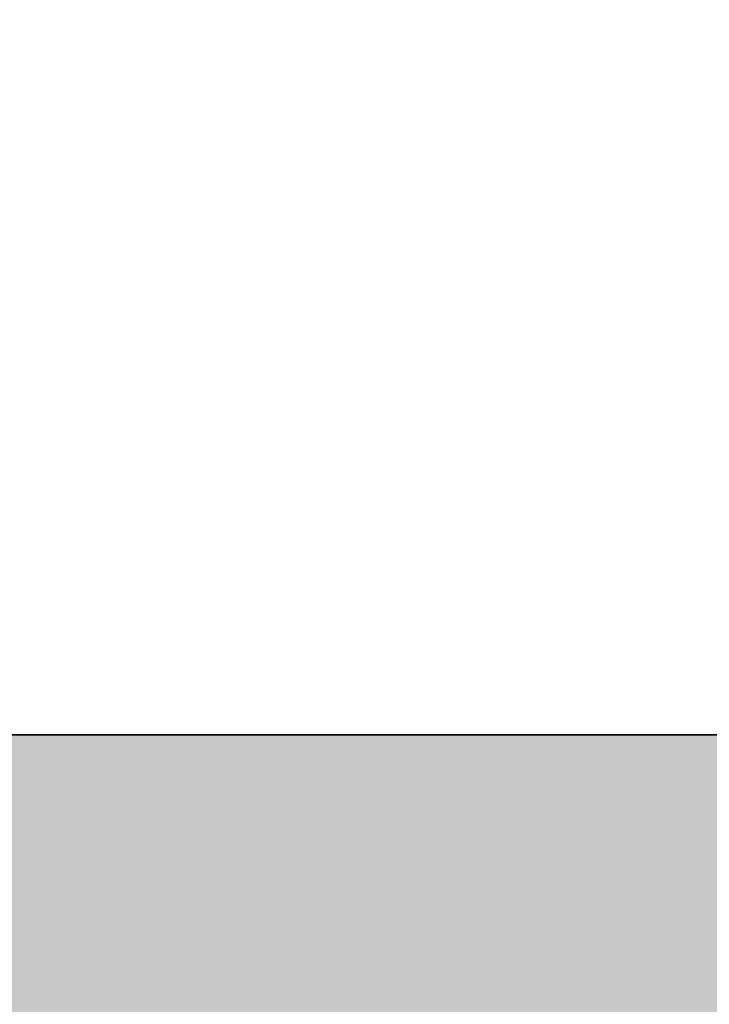
# Model space of a CAD drawing. Units: inches. Extents: x 2696 to 3240, y 1564 to 2310.
# Tile 59 of 76: x 2921.79 to 2936.43, y 2179.88 to 2200.79. Entities that reach past the tile are written whole.
import ezdxf

# ---------------------------------------------------------------- set-up
doc = ezdxf.new("R2010")
doc.units = ezdxf.units.IN
for name, color, linetype, lineweight in [('A-ANNO-DIMS', 3, 'Continuous', 18), ('A-WALL', 7, 'Continuous', 35), ('A-WALL-PATT', 9, 'Continuous', 13)]:
    doc.layers.add(name, color=color, linetype=linetype, lineweight=lineweight)
doc.styles.add('TIMES NEW', font='times.ttf')
doc.dimstyles.new('Siddhuu', dxfattribs={"dimtxt": 6, "dimasz": 2.5, "dimexe": 1.25, "dimexo": 0.625, "dimtad": 1, "dimdec": 1, "dimlunit": 4, "dimtxsty": 'TIMES NEW', "dimcen": 2.5, "dimclrd": 256, "dimclre": 1, "dimclrt": 7, "dimadec": 0, "dimazin": 0, "dimtfac": 1, "dimtdec": 1, "dimtmove": 0, "dimatfit": 3, "dimfxl": 1, "dimtolj": 1, "dimlwd": -1, "dimarcsym": 0})

# ---------------------------------------------------------------- blocks, each defined once
blk = doc.blocks.new('*D59')
at = {"layer": 'A-ANNO-DIMS', "color": 1, "lineweight": -2, "transparency": 16777216}
for p, q in [((2884.709, 1740.826), (2884.709, 2298.451)), ((2956.709, 1740.826), (2956.709, 2298.451))]:
    blk.add_line(p, q, dxfattribs=at)
at = {"layer": 'A-ANNO-DIMS', "transparency": 16777216}
blk.add_line((2887.209, 2297.201), (2954.209, 2297.201), dxfattribs=at)
for points in [[(2887.209, 2297.618), (2887.209, 2296.784), (2884.709, 2297.201)], [(2954.209, 2297.618), (2954.209, 2296.784), (2956.709, 2297.201)]]:
    blk.add_solid(points, dxfattribs=at)
at = {"layer": 'Defpoints', "color": 0, "transparency": 16777216}
for p in [(2956.709, 2297.201), (2884.709, 1740.201), (2956.709, 1740.201)]:
    blk.add_point(p, dxfattribs=at)
at = {"layer": 'A-ANNO-DIMS', "color": 7, "transparency": 16777216, "insert": (2920.709, 2300.878), "char_height": 6, "attachment_point": 5, "style": 'TIMES NEW'}
blk.add_mtext('\\A1;6\'-0"', dxfattribs=at)
blk = doc.blocks.new('*D64')
at = {"layer": 'A-ANNO-DIMS', "color": 1, "lineweight": -2, "transparency": 16777216}
for p, q in [((3073.084, 2206.701), (2709.361, 2206.701)), ((3068.584, 1989.201), (2709.361, 1989.201))]:
    blk.add_line(p, q, dxfattribs=at)
at = {"layer": 'A-ANNO-DIMS', "transparency": 16777216}
blk.add_line((2710.611, 1991.701), (2710.611, 2204.201), dxfattribs=at)
for points in [[(2710.195, 2204.201), (2711.028, 2204.201), (2710.611, 2206.701)], [(2710.195, 1991.701), (2711.028, 1991.701), (2710.611, 1989.201)]]:
    blk.add_solid(points, dxfattribs=at)
at = {"layer": 'Defpoints', "color": 0, "transparency": 16777216}
for p in [(2710.611, 2206.701), (3073.709, 2206.701), (3069.209, 1989.201)]:
    blk.add_point(p, dxfattribs=at)
at = {"layer": 'A-ANNO-DIMS', "color": 7, "transparency": 16777216, "insert": (2706.85, 2097.951), "char_height": 6, "attachment_point": 5, "rotation": 90, "style": 'TIMES NEW'}
blk.add_mtext('\\A1;18\'-1 1/2"', dxfattribs=at)

msp = doc.modelspace()

# ---------------------------------------------------------------- hatches: boundary and pattern name
at = {"layer": 'A-WALL-PATT', "transparency": 33554556}
h = msp.add_hatch(color=256, dxfattribs=at)
h.dxf.hatch_style = 1
h.paths.add_polyline_path([(2879.111, 2253.201), (2905.91, 2253.201), (2905.91, 2262.201), (2841.889, 2262.201), (2841.889, 2253.201), (2870.111, 2253.201), (2870.111, 2176.601), (2965.709, 2176.601), (2965.709, 2206.701), (2973.583, 2206.701), (2973.583, 2215.701), (2965.709, 2215.701), (2965.709, 2262.201), (2929.91, 2262.201), (2929.91, 2253.201), (2956.709, 2253.201), (2956.709, 2185.601), (2879.111, 2185.601)])
h.paths.add_polyline_path([(2782.834, 2262.201), (2745.611, 2262.201), (2745.611, 2228.729), (2754.611, 2228.729), (2754.611, 2253.201), (2782.834, 2253.201)])
h.paths.add_polyline_path([(2754.611, 2136.201), (2965.709, 2136.201), (2965.709, 2145.201), (2879.111, 2145.201), (2879.111, 2147.074), (2877.34, 2147.074), (2870.111, 2147.074), (2870.111, 2145.201), (2754.611, 2145.201), (2754.611, 2169.674), (2745.611, 2169.674), (2745.611, 2000.201), (2754.611, 2000.201), (2754.611, 2019.201), (2849.083, 2019.201), (2849.083, 2023.701), (2841.209, 2023.701), (2841.209, 2051.827), (2836.709, 2051.827), (2836.709, 2023.701), (2754.611, 2023.701), (2754.611, 2091.201), (2836.709, 2091.201), (2836.709, 2087.827), (2841.209, 2087.827), (2841.209, 2095.701), (2754.611, 2095.701)])
h.paths.add_polyline_path([(2965.709, 2136.201), (2956.709, 2136.201), (2956.709, 2023.701), (2885.083, 2023.701), (2885.083, 2019.201), (2956.709, 2019.201), (2956.709, 1950.575), (2965.709, 1950.575), (2965.709, 1980.201), (2973.583, 1980.201), (2973.583, 1989.201), (2965.709, 1989.201)])
h.paths.add_polyline_path([(2754.611, 1906.701), (2880.209, 1906.701), (2884.709, 1906.701), (2956.709, 1906.701), (2956.709, 1792.701), (2944.709, 1792.701), (2944.709, 1783.701), (2956.709, 1783.701), (2956.709, 1740.201), (2884.709, 1740.201), (2884.709, 1783.701), (2896.709, 1783.701), (2896.709, 1792.701), (2884.709, 1792.701), (2884.709, 1846.701), (2880.209, 1846.701), (2880.209, 1740.201), (2754.611, 1740.201), (2754.611, 1777.201), (2745.611, 1777.201), (2745.611, 1692.701), (2754.611, 1692.701), (2754.611, 1731.201), (2956.709, 1731.201), (2956.709, 1723.327), (2965.709, 1723.327), (2965.709, 1884.201), (2973.583, 1884.201), (2973.583, 1893.201), (2965.709, 1893.201), (2965.709, 1914.575), (2956.709, 1914.575), (2956.709, 1911.201), (2754.611, 1911.201), (2754.611, 1930.201), (2745.611, 1930.201), (2745.611, 1817.201), (2754.611, 1817.201), (2754.611, 1854.201), (2826.611, 1854.201), (2826.611, 1868.827), (2822.111, 1868.827), (2822.111, 1858.701), (2754.611, 1858.701)])
h.paths.add_polyline_path([(2965.709, 1656.201), (3008.237, 1656.201), (3008.237, 1665.201), (2965.709, 1665.201), (2965.709, 1693.327), (2956.709, 1693.327), (2956.709, 1686.201), (2934.583, 1686.201), (2934.583, 1681.701), (2956.709, 1681.701), (2956.709, 1614.201), (2896.709, 1614.201), (2896.709, 1681.701), (2904.583, 1681.701), (2904.583, 1686.201), (2892.209, 1686.201), (2892.209, 1614.201), (2858.41, 1614.201), (2858.41, 1605.201), (2965.709, 1605.201)])
h.paths.add_polyline_path([(2788.41, 1614.201), (2754.611, 1614.201), (2754.611, 1652.701), (2745.611, 1652.701), (2745.611, 1605.201), (2788.41, 1605.201)])
h.paths.add_polyline_path([(3199.611, 1633.048), (3190.611, 1633.048), (3190.611, 1614.201), (3082.611, 1614.201), (3082.611, 1665.201), (3070.237, 1665.201), (3070.237, 1656.201), (3078.111, 1656.201), (3078.111, 1605.201), (3199.611, 1605.201)])
h.paths.add_polyline_path([(3199.611, 1702.048), (3190.611, 1702.048), (3190.611, 1699.701), (3106.611, 1699.701), (3106.611, 1747.701), (3190.611, 1747.701), (3190.611, 1752.201), (3082.611, 1752.201), (3082.611, 1760.075), (3078.111, 1760.075), (3078.111, 1747.701), (3102.111, 1747.701), (3102.111, 1699.701), (3078.111, 1699.701), (3078.111, 1695.201), (3190.611, 1695.201), (3190.611, 1676.355), (3199.611, 1676.355)])
h.paths.add_polyline_path([(3199.611, 1783.201), (3190.611, 1783.201), (3190.611, 1745.355), (3199.611, 1745.355)])
h.paths.add_polyline_path([(3082.611, 1884.201), (3190.611, 1884.201), (3190.611, 1853.201), (3199.611, 1853.201), (3199.611, 1901.701), (3190.611, 1901.701), (3190.611, 1893.201), (3005.583, 1893.201), (3005.583, 1891.281), (3005.583, 1884.201), (3078.111, 1884.201), (3078.111, 1792.075), (3082.611, 1792.075)])
h.paths.add_polyline_path([(3199.611, 1994.701), (3190.611, 1994.701), (3190.611, 1989.201), (3073.709, 1989.201), (3073.709, 2034.201), (3069.209, 2034.201), (3069.209, 1989.201), (3005.583, 1989.201), (3005.583, 1980.201), (3190.611, 1980.201), (3190.611, 1971.701), (3199.611, 1971.701)])
h.paths.add_polyline_path([(3199.611, 2155.201), (3190.611, 2155.201), (3190.611, 2064.701), (3199.611, 2064.701)])
h.paths.add_polyline_path([(3190.611, 2074.701), (3106.611, 2074.701), (3106.611, 2122.701), (3190.611, 2122.701), (3190.611, 2127.201), (3082.709, 2127.201), (3082.709, 2135.075), (3073.709, 2135.075), (3073.709, 2122.701), (3102.111, 2122.701), (3102.111, 2074.701), (3069.209, 2074.701), (3069.209, 2070.201), (3190.611, 2070.201)])
h.paths.add_polyline_path([(3082.709, 2253.201), (3190.611, 2253.201), (3190.611, 2225.201), (3199.611, 2225.201), (3199.611, 2262.201), (3073.709, 2262.201), (3073.709, 2215.701), (3035.583, 2215.701), (3035.583, 2206.701), (3073.709, 2206.701), (3073.709, 2171.075), (3082.709, 2171.075)])

# ---------------------------------------------------------------- linework, layer by layer
at = {"layer": 'A-WALL'}
msp.add_line((2879.111, 2185.601), (2956.709, 2185.601), dxfattribs=at)

# ---------------------------------------------------------------- dimensions: what is measured, and where the dimension line sits
at = {"layer": 'A-ANNO-DIMS'}
dim = msp.add_linear_dim(base=(2956.709, 2297.201), p1=(2884.709, 1740.201), p2=(2956.709, 1740.201), dimstyle='Siddhuu', override={"dimdec": 1, "dimlfac": 1, "dimrnd": 0, "dimzin": 1, "dimdsep": 46, "dimlunit": 4, "dimfrac": 2}, dxfattribs=at)
dim.commit()
dim.dimension.update_dxf_attribs({"geometry": '*D59', "text_midpoint": (2920.709, 2300.878)})
dim = msp.add_linear_dim(base=(2710.611, 2206.701), p1=(3069.209, 1989.201), p2=(3073.709, 2206.701), angle=90, dimstyle='Siddhuu', override={"dimdec": 1, "dimlfac": 1, "dimrnd": 0, "dimzin": 1, "dimdsep": 46, "dimlunit": 4, "dimfrac": 2}, dxfattribs=at)
dim.commit()
dim.dimension.update_dxf_attribs({"geometry": '*D64', "text_midpoint": (2706.85, 2097.951)})

doc.saveas('drawing.dxf')
